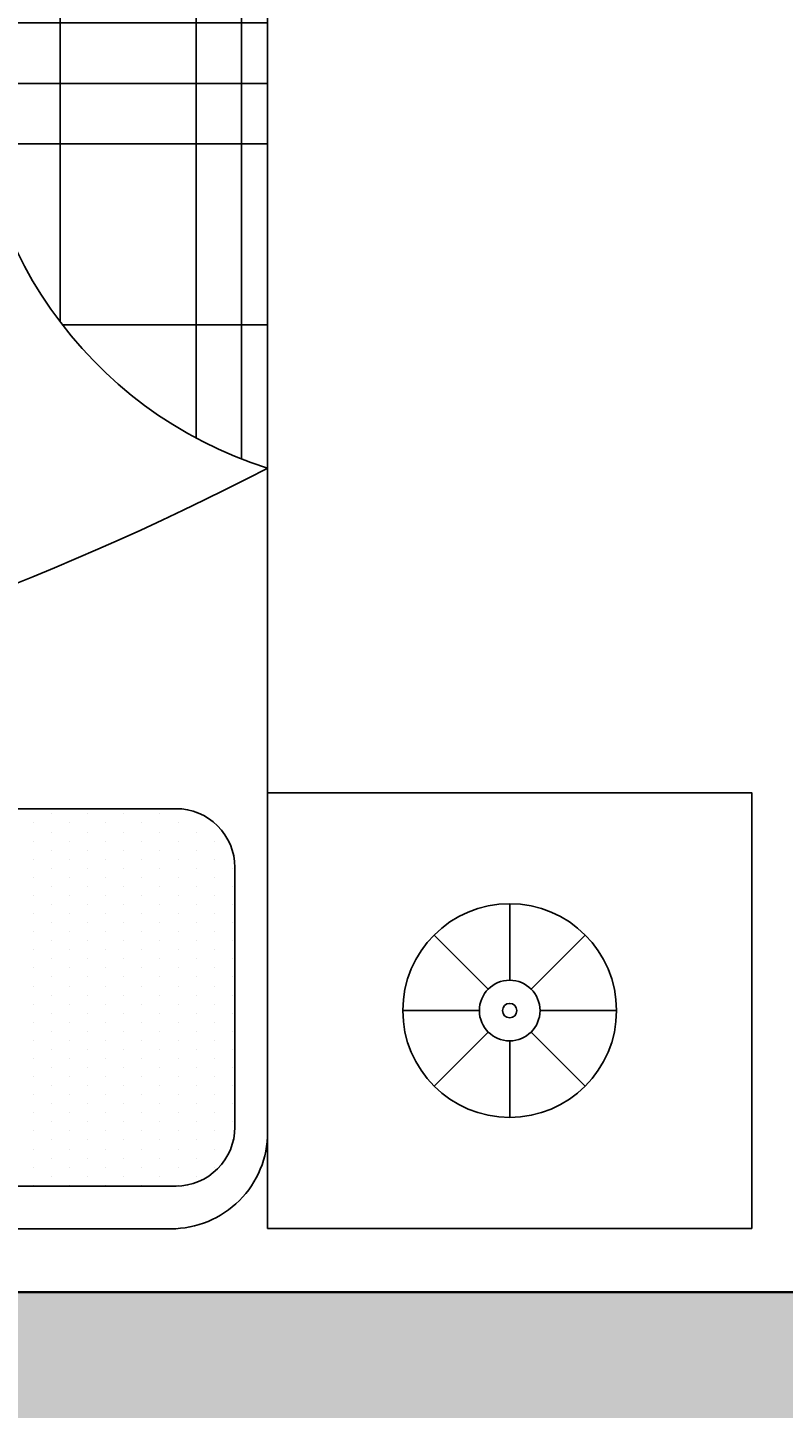
# Model space of a CAD drawing. Units: millimetres. Extents: x 2817 to 5038, y 1110 to 3565.
# Tile 15 of 21: x 2917 to 2946, y 1505 to 1558. Entities that reach past the tile are written whole.
import ezdxf

# ---------------------------------------------------------------- set-up
doc = ezdxf.new("R2010")
doc.units = ezdxf.units.MM
for name, color, linetype, lineweight in [('A-ANNO-DIMS', 2, 'Continuous', 18), ('A-WALL', 7, 'Continuous', 35), ('FURNITURE', 219, 'Continuous', 18)]:
    doc.layers.add(name, color=color, linetype=linetype, lineweight=lineweight)
doc.layers.add('A-WALL-PATT', color=51, linetype='Continuous', lineweight=13, true_color=0xf7f281)
doc.layers.add('BLOCK', color=6, linetype='Continuous')
doc.styles.get("Standard").update_dxf_attribs({"font": 'arial.ttf'})
doc.dimstyles.get("Standard").update_dxf_attribs({"dimtxt": 0.18, "dimasz": 0.18, "dimexe": 0.18, "dimexo": 0.0625, "dimgap": 0.09, "dimtad": 0, "dimtih": 1, "dimtoh": 1, "dimdec": 4, "dimzin": 0, "dimdsep": 46, "dimtxsty": 'Standard', "dimcen": 0.09, "dimadec": 0, "dimazin": 0, "dimtfac": 1, "dimtdec": 4, "dimtofl": 0, "dimtmove": 0, "dimatfit": 3, "dimfxl": 1, "dimtolj": 1, "dimtzin": 0, "dimarcsym": 0})

# ---------------------------------------------------------------- blocks, each defined once
blk = doc.blocks.new('*X7')
at = {"color": 0}
for p, q in [((276.598, 451.25), (280.51, 451.25)), ((275.455, 450.625), (280.51, 450.625)), ((274.411, 450), (280.51, 450)), ((265.51, 448.125), (267.634, 448.125)), ((271.723, 448.125), (280.51, 448.125)), ((265.51, 446.25), (268.465, 446.25)), ((269.519, 446.25), (280.51, 446.25)), ((265.51, 445.625), (268.531, 445.625)), ((268.866, 445.625), (280.51, 445.625)), ((265.51, 445), (280.51, 445)), ((265.51, 443.125), (280.51, 443.125)), ((265.51, 441.25), (280.51, 441.25)), ((265.51, 440.625), (280.51, 440.625)), ((265.634, 440), (280.386, 440))]:
    blk.add_line(p, q, dxfattribs=at)
blk = doc.blocks.new('*X8')
at = {"color": 0}
for p, q in [((280.312, 439.886), (280.312, 452.896)), ((278.906, 439.482), (278.906, 452.338)), ((277.5, 439.482), (277.5, 451.702)), ((277.031, 439.482), (277.031, 451.471)), ((276.562, 439.482), (276.562, 451.231)), ((275.156, 439.482), (275.156, 450.451)), ((273.75, 439.482), (273.75, 449.576)), ((265.781, 439.797), (265.781, 449.511)), ((266.25, 439.517), (266.25, 449.296)), ((273.281, 439.482), (273.281, 449.261)), ((272.812, 439.482), (272.812, 448.934)), ((267.656, 439.482), (267.656, 448.095)), ((271.406, 439.482), (271.406, 447.876)), ((270, 439.482), (270, 446.689)), ((269.531, 439.482), (269.531, 446.262)), ((269.062, 439.482), (269.062, 445.817))]:
    blk.add_line(p, q, dxfattribs=at)
blk = doc.blocks.new('*X9')
at = {"color": 0}
for p, q in [((266.4375, 457.03125), (266.4375, 457.03125)), ((266.8125, 457.03125), (266.8125, 457.03125)), ((267.1875, 457.03125), (267.1875, 457.03125)), ((267.5625, 457.03125), (267.5625, 457.03125)), ((267.9375, 457.03125), (267.9375, 457.03125)), ((266.0625, 456.84375), (266.0625, 456.84375)), ((266.25, 456.9375), (266.25, 456.9375)), ((266.4375, 456.84375), (266.4375, 456.84375)), ((266.625, 456.9375), (266.625, 456.9375)), ((266.8125, 456.84375), (266.8125, 456.84375)), ((267, 456.9375), (267, 456.9375)), ((267.1875, 456.84375), (267.1875, 456.84375)), ((267.375, 456.9375), (267.375, 456.9375)), ((267.5625, 456.84375), (267.5625, 456.84375)), ((267.75, 456.9375), (267.75, 456.9375)), ((267.9375, 456.84375), (267.9375, 456.84375)), ((266.25, 456.75), (266.25, 456.75)), ((266.625, 456.75), (266.625, 456.75)), ((267, 456.75), (267, 456.75)), ((267.375, 456.75), (267.375, 456.75)), ((267.75, 456.75), (267.75, 456.75)), ((265.875, 456.5625), (265.875, 456.5625)), ((266.0625, 456.65625), (266.0625, 456.65625)), ((266.25, 456.5625), (266.25, 456.5625)), ((266.4375, 456.65625), (266.4375, 456.65625)), ((266.625, 456.5625), (266.625, 456.5625)), ((266.8125, 456.65625), (266.8125, 456.65625)), ((267, 456.5625), (267, 456.5625)), ((267.1875, 456.65625), (267.1875, 456.65625)), ((267.375, 456.5625), (267.375, 456.5625)), ((267.5625, 456.65625), (267.5625, 456.65625)), ((267.75, 456.5625), (267.75, 456.5625)), ((267.9375, 456.65625), (267.9375, 456.65625)), ((266.0625, 456.46875), (266.0625, 456.46875)), ((266.4375, 456.46875), (266.4375, 456.46875)), ((266.8125, 456.46875), (266.8125, 456.46875)), ((267.1875, 456.46875), (267.1875, 456.46875)), ((267.5625, 456.46875), (267.5625, 456.46875)), ((267.9375, 456.46875), (267.9375, 456.46875)), ((265.875, 456.375), (265.875, 456.375)), ((266.0625, 456.28125), (266.0625, 456.28125)), ((266.25, 456.375), (266.25, 456.375)), ((266.4375, 456.28125), (266.4375, 456.28125)), ((266.625, 456.375), (266.625, 456.375)), ((266.8125, 456.28125), (266.8125, 456.28125)), ((267, 456.375), (267, 456.375)), ((267.1875, 456.28125), (267.1875, 456.28125)), ((267.375, 456.375), (267.375, 456.375)), ((267.5625, 456.28125), (267.5625, 456.28125)), ((267.75, 456.375), (267.75, 456.375)), ((267.9375, 456.28125), (267.9375, 456.28125)), ((265.875, 456.1875), (265.875, 456.1875)), ((266.25, 456.1875), (266.25, 456.1875)), ((266.625, 456.1875), (266.625, 456.1875)), ((267, 456.1875), (267, 456.1875)), ((267.375, 456.1875), (267.375, 456.1875)), ((267.75, 456.1875), (267.75, 456.1875)), ((265.875, 456), (265.875, 456)), ((266.0625, 456.09375), (266.0625, 456.09375)), ((266.25, 456), (266.25, 456)), ((266.4375, 456.09375), (266.4375, 456.09375)), ((266.625, 456), (266.625, 456)), ((266.8125, 456.09375), (266.8125, 456.09375)), ((267, 456), (267, 456)), ((267.1875, 456.09375), (267.1875, 456.09375)), ((267.375, 456), (267.375, 456)), ((267.5625, 456.09375), (267.5625, 456.09375)), ((267.75, 456), (267.75, 456)), ((267.9375, 456.09375), (267.9375, 456.09375)), ((265.875, 455.8125), (265.875, 455.8125)), ((266.0625, 455.90625), (266.0625, 455.90625)), ((266.25, 455.8125), (266.25, 455.8125)), ((266.4375, 455.90625), (266.4375, 455.90625)), ((266.625, 455.8125), (266.625, 455.8125)), ((266.8125, 455.90625), (266.8125, 455.90625)), ((267, 455.8125), (267, 455.8125)), ((267.1875, 455.90625), (267.1875, 455.90625)), ((267.375, 455.8125), (267.375, 455.8125)), ((267.5625, 455.90625), (267.5625, 455.90625)), ((267.75, 455.8125), (267.75, 455.8125)), ((267.9375, 455.90625), (267.9375, 455.90625)), ((266.0625, 455.71875), (266.0625, 455.71875)), ((266.4375, 455.71875), (266.4375, 455.71875)), ((266.8125, 455.71875), (266.8125, 455.71875)), ((267.1875, 455.71875), (267.1875, 455.71875)), ((267.5625, 455.71875), (267.5625, 455.71875)), ((267.9375, 455.71875), (267.9375, 455.71875)), ((265.875, 455.625), (265.875, 455.625)), ((266.0625, 455.53125), (266.0625, 455.53125)), ((266.25, 455.625), (266.25, 455.625)), ((266.4375, 455.53125), (266.4375, 455.53125)), ((266.625, 455.625), (266.625, 455.625)), ((266.8125, 455.53125), (266.8125, 455.53125)), ((267, 455.625), (267, 455.625)), ((267.1875, 455.53125), (267.1875, 455.53125)), ((267.375, 455.625), (267.375, 455.625)), ((267.5625, 455.53125), (267.5625, 455.53125)), ((267.75, 455.625), (267.75, 455.625)), ((267.9375, 455.53125), (267.9375, 455.53125)), ((265.875, 455.4375), (265.875, 455.4375)), ((266.25, 455.4375), (266.25, 455.4375)), ((266.625, 455.4375), (266.625, 455.4375)), ((267, 455.4375), (267, 455.4375)), ((267.375, 455.4375), (267.375, 455.4375)), ((267.75, 455.4375), (267.75, 455.4375)), ((265.875, 455.25), (265.875, 455.25)), ((266.0625, 455.34375), (266.0625, 455.34375)), ((266.25, 455.25), (266.25, 455.25)), ((266.4375, 455.34375), (266.4375, 455.34375)), ((266.625, 455.25), (266.625, 455.25)), ((266.8125, 455.34375), (266.8125, 455.34375)), ((267, 455.25), (267, 455.25)), ((267.1875, 455.34375), (267.1875, 455.34375)), ((267.375, 455.25), (267.375, 455.25)), ((267.5625, 455.34375), (267.5625, 455.34375)), ((267.75, 455.25), (267.75, 455.25)), ((267.9375, 455.34375), (267.9375, 455.34375)), ((266.0625, 455.15625), (266.0625, 455.15625)), ((266.4375, 455.15625), (266.4375, 455.15625)), ((266.8125, 455.15625), (266.8125, 455.15625)), ((267.1875, 455.15625), (267.1875, 455.15625)), ((267.5625, 455.15625), (267.5625, 455.15625)), ((267.9375, 455.15625), (267.9375, 455.15625)), ((265.875, 455.0625), (265.875, 455.0625)), ((266.0625, 454.96875), (266.0625, 454.96875)), ((266.25, 455.0625), (266.25, 455.0625)), ((266.4375, 454.96875), (266.4375, 454.96875)), ((266.625, 455.0625), (266.625, 455.0625)), ((266.8125, 454.96875), (266.8125, 454.96875)), ((267, 455.0625), (267, 455.0625)), ((267.1875, 454.96875), (267.1875, 454.96875)), ((267.375, 455.0625), (267.375, 455.0625)), ((267.5625, 454.96875), (267.5625, 454.96875)), ((267.75, 455.0625), (267.75, 455.0625)), ((267.9375, 454.96875), (267.9375, 454.96875)), ((265.875, 454.875), (265.875, 454.875)), ((266.25, 454.875), (266.25, 454.875)), ((266.625, 454.875), (266.625, 454.875)), ((267, 454.875), (267, 454.875)), ((267.375, 454.875), (267.375, 454.875)), ((267.75, 454.875), (267.75, 454.875)), ((265.875, 454.6875), (265.875, 454.6875)), ((266.0625, 454.78125), (266.0625, 454.78125)), ((266.25, 454.6875), (266.25, 454.6875)), ((266.4375, 454.78125), (266.4375, 454.78125)), ((266.625, 454.6875), (266.625, 454.6875)), ((266.8125, 454.78125), (266.8125, 454.78125)), ((267, 454.6875), (267, 454.6875)), ((267.1875, 454.78125), (267.1875, 454.78125)), ((267.375, 454.6875), (267.375, 454.6875)), ((267.5625, 454.78125), (267.5625, 454.78125)), ((267.75, 454.6875), (267.75, 454.6875)), ((267.9375, 454.78125), (267.9375, 454.78125)), ((266.0625, 454.59375), (266.0625, 454.59375)), ((266.4375, 454.59375), (266.4375, 454.59375)), ((266.8125, 454.59375), (266.8125, 454.59375)), ((267.1875, 454.59375), (267.1875, 454.59375)), ((267.5625, 454.59375), (267.5625, 454.59375)), ((267.9375, 454.59375), (267.9375, 454.59375)), ((265.875, 454.5), (265.875, 454.5)), ((266.0625, 454.40625), (266.0625, 454.40625)), ((266.25, 454.5), (266.25, 454.5)), ((266.4375, 454.40625), (266.4375, 454.40625)), ((266.625, 454.5), (266.625, 454.5)), ((266.8125, 454.40625), (266.8125, 454.40625)), ((267, 454.5), (267, 454.5)), ((267.1875, 454.40625), (267.1875, 454.40625)), ((267.375, 454.5), (267.375, 454.5)), ((267.5625, 454.40625), (267.5625, 454.40625)), ((267.75, 454.5), (267.75, 454.5)), ((267.9375, 454.40625), (267.9375, 454.40625)), ((265.875, 454.3125), (265.875, 454.3125)), ((266.25, 454.3125), (266.25, 454.3125)), ((266.625, 454.3125), (266.625, 454.3125)), ((267, 454.3125), (267, 454.3125)), ((267.375, 454.3125), (267.375, 454.3125)), ((267.75, 454.3125), (267.75, 454.3125)), ((265.875, 454.125), (265.875, 454.125)), ((266.0625, 454.21875), (266.0625, 454.21875)), ((266.25, 454.125), (266.25, 454.125)), ((266.4375, 454.21875), (266.4375, 454.21875)), ((266.625, 454.125), (266.625, 454.125)), ((266.8125, 454.21875), (266.8125, 454.21875)), ((267, 454.125), (267, 454.125)), ((267.1875, 454.21875), (267.1875, 454.21875)), ((267.375, 454.125), (267.375, 454.125)), ((267.5625, 454.21875), (267.5625, 454.21875)), ((267.75, 454.125), (267.75, 454.125)), ((267.9375, 454.21875), (267.9375, 454.21875)), ((266.0625, 454.03125), (266.0625, 454.03125)), ((266.4375, 454.03125), (266.4375, 454.03125)), ((266.8125, 454.03125), (266.8125, 454.03125)), ((267.1875, 454.03125), (267.1875, 454.03125)), ((267.5625, 454.03125), (267.5625, 454.03125)), ((267.9375, 454.03125), (267.9375, 454.03125)), ((265.875, 453.9375), (265.875, 453.9375)), ((266.0625, 453.84375), (266.0625, 453.84375)), ((266.25, 453.9375), (266.25, 453.9375)), ((266.4375, 453.84375), (266.4375, 453.84375)), ((266.625, 453.9375), (266.625, 453.9375)), ((266.8125, 453.84375), (266.8125, 453.84375)), ((267, 453.9375), (267, 453.9375)), ((267.1875, 453.84375), (267.1875, 453.84375)), ((267.375, 453.9375), (267.375, 453.9375)), ((267.5625, 453.84375), (267.5625, 453.84375)), ((267.75, 453.9375), (267.75, 453.9375)), ((267.9375, 453.84375), (267.9375, 453.84375)), ((265.875, 453.75), (265.875, 453.75)), ((266.25, 453.75), (266.25, 453.75)), ((266.625, 453.75), (266.625, 453.75)), ((267, 453.75), (267, 453.75)), ((267.375, 453.75), (267.375, 453.75)), ((267.75, 453.75), (267.75, 453.75)), ((266.0625, 453.65625), (266.0625, 453.65625)), ((266.25, 453.5625), (266.25, 453.5625)), ((266.4375, 453.65625), (266.4375, 453.65625)), ((266.625, 453.5625), (266.625, 453.5625)), ((266.8125, 453.65625), (266.8125, 453.65625)), ((267, 453.5625), (267, 453.5625)), ((267.1875, 453.65625), (267.1875, 453.65625)), ((267.375, 453.5625), (267.375, 453.5625)), ((267.5625, 453.65625), (267.5625, 453.65625)), ((267.75, 453.5625), (267.75, 453.5625)), ((267.9375, 453.65625), (267.9375, 453.65625)), ((266.0625, 453.46875), (266.0625, 453.46875)), ((266.4375, 453.46875), (266.4375, 453.46875)), ((266.8125, 453.46875), (266.8125, 453.46875)), ((267.1875, 453.46875), (267.1875, 453.46875)), ((267.5625, 453.46875), (267.5625, 453.46875)), ((267.9375, 453.46875), (267.9375, 453.46875)), ((266.0625, 453.28125), (266.0625, 453.28125)), ((266.25, 453.375), (266.25, 453.375)), ((266.4375, 453.28125), (266.4375, 453.28125)), ((266.625, 453.375), (266.625, 453.375)), ((266.8125, 453.28125), (266.8125, 453.28125)), ((267, 453.375), (267, 453.375)), ((267.1875, 453.28125), (267.1875, 453.28125)), ((267.375, 453.375), (267.375, 453.375)), ((267.5625, 453.28125), (267.5625, 453.28125)), ((267.75, 453.375), (267.75, 453.375)), ((267.9375, 453.28125), (267.9375, 453.28125)), ((266.25, 453.1875), (266.25, 453.1875)), ((266.625, 453.1875), (266.625, 453.1875)), ((267, 453.1875), (267, 453.1875)), ((267.375, 453.1875), (267.375, 453.1875)), ((267.75, 453.1875), (267.75, 453.1875))]:
    blk.add_line(p, q, dxfattribs=at)
blk = doc.blocks.new('A$C52E67D0D')
at = {"layer": 'BLOCK'}
for p, q in [((250.5, 1605.5), (250.5, 1684.7)), ((228.3, 1596.3), (172.3, 1652.3)), ((272.7, 1596.3), (328.7, 1652.3)), ((219.1, 1574.1), (139.9, 1574.1)), ((281.9, 1574.1), (361.1, 1574.1)), ((228.3, 1551.9), (172.3, 1495.9)), ((272.7, 1551.9), (328.7, 1495.9)), ((250.5, 1542.8), (250.5, 1463.5))]:
    blk.add_line(p, q, dxfattribs=at)
blk.add_lwpolyline([(501, 1348.6), (501, 1799.6), (0, 1799.6), (0, 1348.6)], close=True, dxfattribs=at)
for points in [[(1901, 0), (601, 0, -0.414214), (501, 100), (501, 1700, -0.414214), (601, 1800), (1901, 1800, -0.414214), (2001, 1700), (2001, 100, -0.414214)], [(1171.8, 1365.1), (595.8, 1365.1, -0.414214), (535, 1425.9), (535, 1694.8, -0.414214), (595.8, 1755.7), (1171.8, 1755.7, -0.414214), (1232.6, 1694.8), (1232.6, 1425.9, -0.414214)]]:
    blk.add_lwpolyline(points, format="xyb", close=True, dxfattribs=at)
for radius in [110.6, 31.4, 7.46]:
    blk.add_circle((250.5, 1574.1), radius, dxfattribs=at)
for centre, radius, start, end in [((1888.6, -1664.5), 3015.3, 87.8642, 117.4001), ((371.4, 600.4), 432, 357.3792, 72.5379)]:
    blk.add_arc(centre, radius, start, end, dxfattribs=at)
at = {"layer": 'BLOCK', "xscale": 100, "yscale": 100, "zscale": 100}
for name in ['*X9', '*X8', '*X7']:
    blk.add_blockref(name, (-26050, -43948.2), dxfattribs=at)
blk = doc.blocks.new('*D38')
at = {"layer": 'A-ANNO-DIMS', "color": 0, "lineweight": -2, "transparency": 16777216}
for p, q in [((3110.177, 1573.436), (2817.308, 1573.436)), ((2817.488, 1573.256), (2817.488, 1523.618)), ((2817.488, 1473.616), (2817.488, 1523.254)), ((3105.677, 1473.436), (2817.308, 1473.436))]:
    blk.add_line(p, q, dxfattribs=at)
for points in [[(2817.458, 1573.256), (2817.518, 1573.256), (2817.488, 1573.436)], [(2817.458, 1473.616), (2817.518, 1473.616), (2817.488, 1473.436)]]:
    blk.add_solid(points, dxfattribs=at)
at = {"layer": 'Defpoints', "color": 0, "lineweight": -2, "transparency": 16777216}
for p in [(2817.488, 1573.436), (3110.239, 1573.436), (3105.739, 1473.436)]:
    blk.add_point(p, dxfattribs=at)
at = {"layer": 'A-ANNO-DIMS', "color": 0, "transparency": 16777216, "insert": (2817.488, 1523.436), "char_height": 0.18, "attachment_point": 5}
blk.add_mtext('\\A1;100', dxfattribs=at)

msp = doc.modelspace()

# ---------------------------------------------------------------- hatches: boundary and pattern name
at = {"layer": 'A-WALL-PATT'}
h = msp.add_hatch(color=256, dxfattribs=at)
h.dxf.hatch_style = 1
h.paths.add_polyline_path([(3061.2393, 1549.7835), (3052.2393, 1549.7835), (3052.2393, 1509.4357), (2991.7393, 1509.4357), (2991.7393, 1575.4357), (2982.7393, 1575.4357), (2982.7393, 1509.4357), (2982.7393, 1500.4357), (3052.2393, 1500.4357), (3052.2393, 1498.4661), (3061.2393, 1498.613)])
h.paths.add_polyline_path([(2946.7393, 1505.8357), (2946.7393, 1509.4357), (2850.7393, 1509.4357), (2850.7393, 1520.7609), (2841.7393, 1520.7609), (2841.7393, 1427.2177), (2850.7393, 1427.3646), (2850.7393, 1500.4357), (2922.7393, 1500.4357), (2931.7393, 1500.4357), (2946.7393, 1500.4357)])
h.paths.add_polyline_path([(3061.2393, 1450.613), (3052.2393, 1450.613), (3052.2393, 1431.4357), (3059.4393, 1431.4357), (3061.2393, 1431.4357)])
h.paths.add_polyline_path([(3061.2393, 1211.2899), (3052.2393, 1211.2899), (3052.2393, 1195.4357), (3059.4393, 1195.4357), (3061.2393, 1195.4357)])

# ---------------------------------------------------------------- linework, layer by layer
at = {"layer": 'A-WALL'}
msp.add_line((2850.7393, 1509.4357), (2946.7393, 1509.4357), dxfattribs=at)

# ---------------------------------------------------------------- block references
at = {"layer": 'FURNITURE', "xscale": 0.0367705835331598, "yscale": 0.0367705835331598, "zscale": 0.0367705835331598, "rotation": 180}
msp.add_blockref('A$C52E67D0D', (2944.3285, 1578.0385), dxfattribs=at)

# ---------------------------------------------------------------- dimensions: what is measured, and where the dimension line sits
at = {"layer": 'A-ANNO-DIMS'}
dim = msp.add_linear_dim(base=(2817.4881, 1573.4357), p1=(3105.7393, 1473.4357), p2=(3110.2393, 1573.4357), angle=90, dimstyle='Standard', override={"dimdec": 0, "dimlfac": 1, "dimrnd": 0, "dimzin": 0, "dimdsep": 46, "dimlunit": 2}, dxfattribs=at)
dim.commit()
dim.dimension.update_dxf_attribs({"geometry": '*D38', "text_midpoint": (2817.4881, 1523.4357)})

doc.saveas('drawing.dxf')
